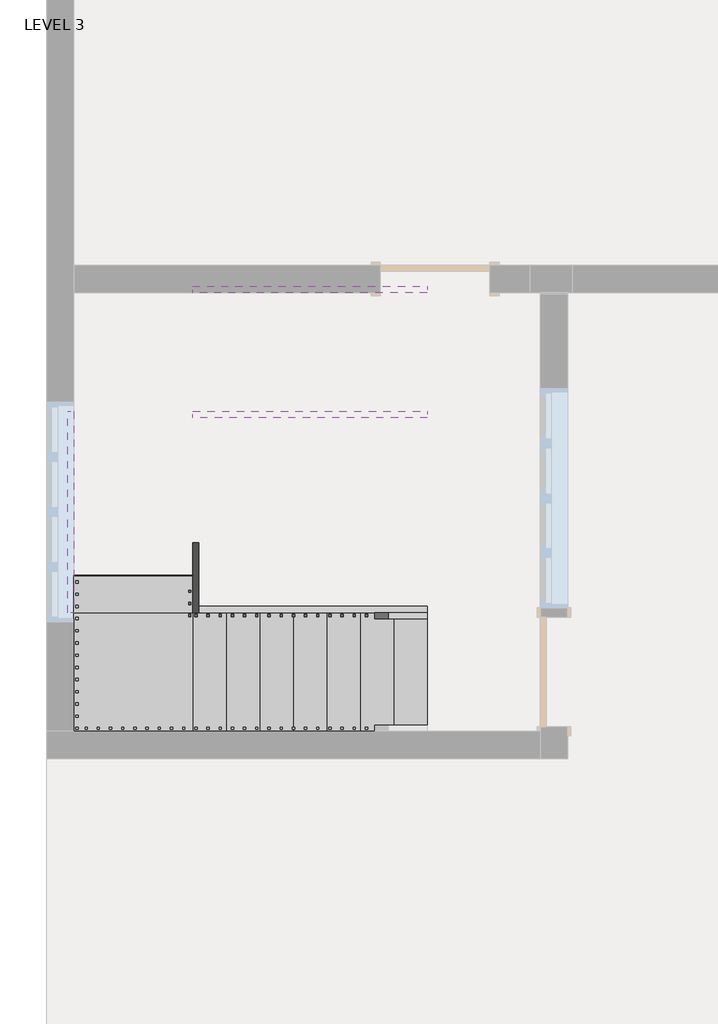
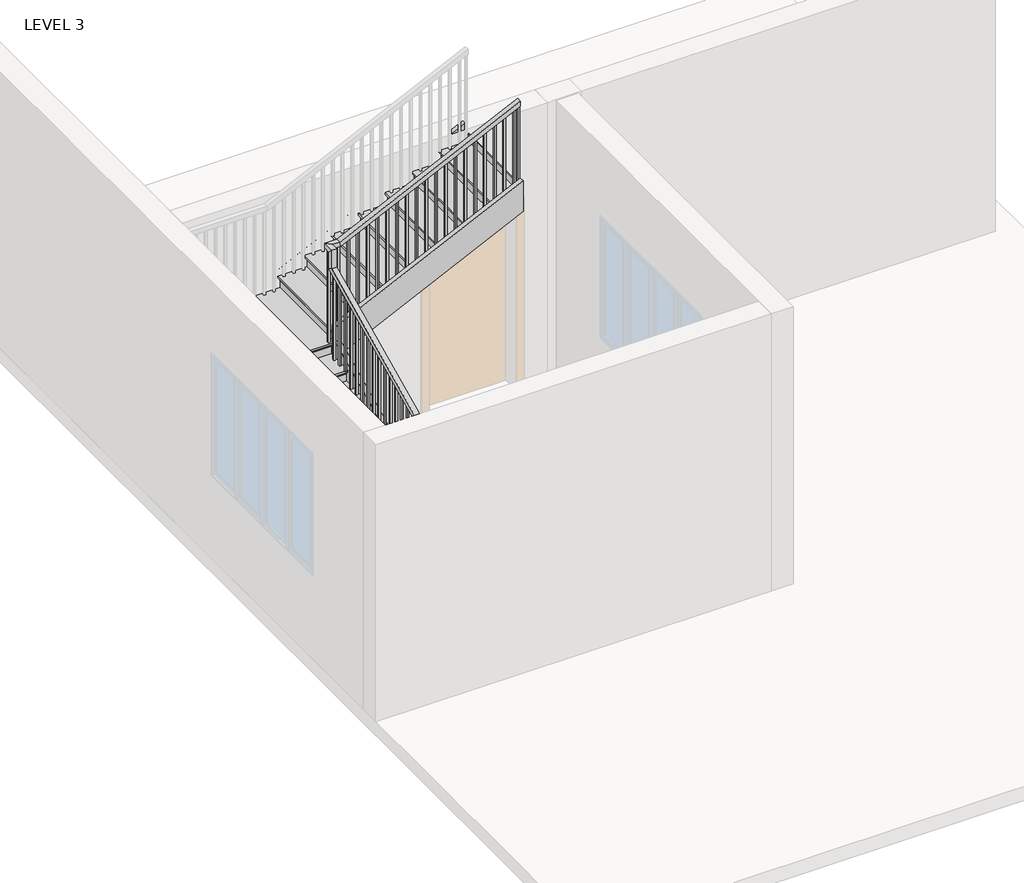
# One storey, part 3 of 3: 6 members, 1 railing, 1 stair flight.
"""IFC4 building model written with IfcOpenShell, lengths in millimetres."""

from ifc_helpers import new_model, si_unit, frame, origin, place, context, project, spatial, polyline, outline, extrude, faceted_brep, transform, mapped, element, save
from components import stair_flight_8adf14a6

model = new_model("IFC4")

# Units and contexts
model_context = context("Model", 3, world=origin())
ifc_project = project(units=[si_unit("LENGTHUNIT", "METRE", prefix="MILLI")], contexts=[model_context])

# Site, building, storey
site = spatial("IfcSite", under=ifc_project)
building = spatial("IfcBuilding", under=site)
storey = spatial("IfcBuildingStorey", under=building, Name="LEVEL 3", Elevation=6248.4)

# Members
placement = place(None, origin())
element("IfcMember", 1, ObjectType="Stringer - 2\" Width", at=placement, inside=storey, context=model_context, shape_type="SweptSolid", body=[
    extrude(outline(polyline([(6248.4, -19769.8789184), (6449.6074226, -19769.8789184), (7039.9315333, -21014.4789184), (7039.9315333, -21725.7197387), (6248.4, -20056.9074227), (6248.4, -19769.8789184)])), frame((0.0, -1169.2399287, 0.0), z_axis=(0.0, 1.0, 0.0), x_axis=(0.0, 0.0, 1.0)), (0.0, 0.0, 1.0), 50.8),
])
element("IfcMember", 2, ObjectType="Stringer - 2\" Width", at=placement, inside=storey, context=model_context, shape_type="SweptSolid", body=[
    extrude(outline(polyline([(-127.880749, 7509.7619743), (837.3600713, 7967.5837072), (1548.6008915, 7967.5837072), (583.3600713, 7509.7619743), (-127.880749, 7509.7619743)])), frame((-22767.0789184, 0.0, 0.0), z_axis=(1.0, 0.0, 0.0), x_axis=(0.0, 1.0, 0.0)), (0.0, 0.0, 1.0), 50.8),
])
element("IfcMember", 3, ObjectType="Stringer - 2\" Width", at=placement, inside=storey, context=model_context, shape_type="SweptSolid", body=[
    extrude(outline(polyline([(8437.4141482, -21014.4789184), (9027.7382589, -19769.8789184), (9365.0856835, -19769.8789184), (8437.4141482, -21725.7197387), (8437.4141482, -21014.4789184)])), frame((0.0, 2539.1600713, 0.0), z_axis=(0.0, 1.0, 0.0), x_axis=(0.0, 0.0, 1.0)), (0.0, 0.0, 1.0), 50.8),
])
element("IfcMember", 4, ObjectType="Stringer - 2\" Width", at=placement, inside=storey, context=model_context, shape_type="SweptSolid", body=[
    extrude(outline(polyline([(6248.4, -19769.8789184), (6449.6074226, -19769.8789184), (7353.1647349, -21674.8789184), (7015.8173103, -21674.8789184), (6248.4, -20056.9074227), (6248.4, -19769.8789184)])), frame((0.0, -127.8399287, 0.0), z_axis=(0.0, 1.0, 0.0), x_axis=(0.0, 0.0, 1.0)), (0.0, 0.0, 1.0), 50.8),
])
element("IfcMember", 5, ObjectType="Stringer - 2\" Width", at=placement, inside=storey, context=model_context, shape_type="SweptSolid", body=[
    extrude(outline(polyline([(-127.8399287, 7172.433911), (-127.8399287, 7509.7813357), (1497.7600713, 8280.8169088), (1497.7600713, 7943.4694842), (-127.8399287, 7172.433911)])), frame((-21725.6789184, 0.0, 0.0), z_axis=(1.0, 0.0, 0.0), x_axis=(0.0, 1.0, 0.0)), (0.0, 0.0, 1.0), 50.8),
])
element("IfcMember", 6, ObjectType="Stringer - 2\" Width", at=placement, inside=storey, context=model_context, shape_type="SweptSolid", body=[
    extrude(outline(polyline([(8437.4335096, -21725.6789184), (8100.086085, -21725.6789184), (9027.7382589, -19769.8789184), (9365.0856835, -19769.8789184), (8437.4335096, -21725.6789184)])), frame((0.0, 1497.7600713, 0.0), z_axis=(0.0, 1.0, 0.0), x_axis=(0.0, 0.0, 1.0)), (0.0, 0.0, 1.0), 50.8),
])

# Railing
element("IfcRailing", 7, ObjectType="Handrail - Rectangular", at=placement, inside=storey, context=model_context, shape_type="SolidModel", body=[
    faceted_brep([(-19769.8789184, -178.6399287, 7295.3217391), (-19769.8789184, -178.6399287, 7239.0971684), (-19769.8789184, -127.8399287, 7239.0971684), (-19769.8789184, -127.8399287, 7295.3217391), (-21649.4789184, -178.6399287, 8186.8316206), (-21700.2789184, -178.6399287, 8154.7019114), (-21700.2789184, -127.8399287, 8154.7019114), (-21649.4789184, -127.8399287, 8186.8316206), (-21776.4789184, -40.2031254, 8340.8379447), (-21776.4789184, -51.6399287, 8391.6379447), (-21776.4789184, 1472.3600713, 9114.4837945), (-21776.4789184, 1523.1600713, 9082.3540854), (-21725.6789184, -40.2031254, 8340.8379447), (-21725.6789184, 1523.1600713, 9082.3540854), (-21725.6789184, -51.6399287, 8391.6379447), (-21725.6789184, 1472.3600713, 9114.4837945), (-19769.8789184, 1599.3600713, 10210.8), (-19769.8789184, 1548.5600713, 10210.8), (-19769.8789184, 1548.5600713, 10154.5754292), (-19769.8789184, 1599.3600713, 10154.5754292), (-21638.0421151, 1599.3600713, 9268.4901186), (-21649.4789184, 1599.3600713, 9319.2901186), (-21638.0421151, 1548.5600713, 9268.4901186), (-21649.4789184, 1548.5600713, 9319.2901186), (-21649.4789184, -178.6399287, 8391.6379447), (-21700.2789184, -178.6399287, 8340.8379447), (-21700.2789184, -127.8399287, 8340.8379447), (-21649.4789184, -127.8399287, 8391.6379447), (-21776.4789184, -178.6399287, 8391.6379447), (-21776.4789184, -178.6399287, 8340.8379447), (-21725.6789184, -127.8399287, 8340.8379447), (-21725.6789184, -127.8399287, 8391.6379447), (-21776.4789184, 1472.3600713, 9319.2901186), (-21776.4789184, 1523.1600713, 9268.4901186), (-21725.6789184, 1523.1600713, 9268.4901186), (-21725.6789184, 1472.3600713, 9319.2901186), (-21776.4789184, 1599.3600713, 9319.2901186), (-21776.4789184, 1599.3600713, 9268.4901186), (-21725.6789184, 1548.5600713, 9268.4901186), (-21725.6789184, 1548.5600713, 9319.2901186)], [[[0, 1, 2, 3]], [[1, 0, 4, 5]], [[2, 1, 5, 6]], [[3, 2, 6, 7]], [[0, 3, 7, 4]], [[8, 9, 10, 11]], [[12, 8, 11, 13]], [[14, 12, 13, 15]], [[9, 14, 15, 10]], [[16, 17, 18, 19]], [[20, 21, 16, 19]], [[22, 20, 19, 18]], [[23, 22, 18, 17]], [[21, 23, 17, 16]], [[5, 4, 24, 25]], [[6, 5, 25, 26]], [[7, 6, 26, 27]], [[4, 7, 27, 24]], [[25, 24, 28, 29]], [[26, 25, 29, 30]], [[27, 26, 30, 31]], [[24, 27, 31, 28]], [[29, 28, 9, 8]], [[30, 29, 8, 12]], [[31, 30, 12, 14]], [[28, 31, 14, 9]], [[11, 10, 32, 33]], [[13, 11, 33, 34]], [[15, 13, 34, 35]], [[10, 15, 35, 32]], [[33, 32, 36, 37]], [[34, 33, 37, 38]], [[35, 34, 38, 39]], [[32, 35, 39, 36]], [[37, 36, 21, 20]], [[38, 37, 20, 22]], [[39, 38, 22, 23]], [[36, 39, 23, 21]]]),
    extrude(outline(polyline([(10134.9983541, -19811.1539184), (10125.962781, -19830.2039184), (9163.8782609, -19830.2039184), (9163.8782609, -19811.1539184), (10134.9983541, -19811.1539184)])), frame((0.0, 1564.4350713, 0.0), z_axis=(0.0, 1.0, 0.0), x_axis=(0.0, 0.0, 1.0)), (0.0, 0.0, 1.0), 19.05),
    extrude(outline(polyline([(10086.8086308, -19912.7539184), (10077.7730577, -19931.8039184), (9163.8782609, -19931.8039184), (9163.8782609, -19912.7539184), (10086.8086308, -19912.7539184)])), frame((0.0, 1564.4350713, 0.0), z_axis=(0.0, 1.0, 0.0), x_axis=(0.0, 0.0, 1.0)), (0.0, 0.0, 1.0), 19.05),
    extrude(outline(polyline([(10038.6189075, -20014.3539184), (10029.5833344, -20033.4039184), (9163.8782609, -20033.4039184), (9163.8782609, -20014.3539184), (10038.6189075, -20014.3539184)])), frame((0.0, 1564.4350713, 0.0), z_axis=(0.0, 1.0, 0.0), x_axis=(0.0, 0.0, 1.0)), (0.0, 0.0, 1.0), 19.05),
    extrude(outline(polyline([(9990.4291842, -20115.9539184), (9981.393611, -20135.0039184), (9031.3565217, -20135.0039184), (9031.3565217, -20115.9539184), (9990.4291842, -20115.9539184)])), frame((0.0, 1564.4350713, 0.0), z_axis=(0.0, 1.0, 0.0), x_axis=(0.0, 0.0, 1.0)), (0.0, 0.0, 1.0), 19.05),
    extrude(outline(polyline([(9942.2394608, -20217.5539184), (9933.2038877, -20236.6039184), (9031.3565217, -20236.6039184), (9031.3565217, -20217.5539184), (9942.2394608, -20217.5539184)])), frame((0.0, 1564.4350713, 0.0), z_axis=(0.0, 1.0, 0.0), x_axis=(0.0, 0.0, 1.0)), (0.0, 0.0, 1.0), 19.05),
    extrude(outline(polyline([(9894.0497375, -20319.1539184), (9885.0141644, -20338.2039184), (9031.3565217, -20338.2039184), (9031.3565217, -20319.1539184), (9894.0497375, -20319.1539184)])), frame((0.0, 1564.4350713, 0.0), z_axis=(0.0, 1.0, 0.0), x_axis=(0.0, 0.0, 1.0)), (0.0, 0.0, 1.0), 19.05),
    extrude(outline(polyline([(9845.8600142, -20420.7539184), (9836.8244411, -20439.8039184), (8898.8347826, -20439.8039184), (8898.8347826, -20420.7539184), (9845.8600142, -20420.7539184)])), frame((0.0, 1564.4350713, 0.0), z_axis=(0.0, 1.0, 0.0), x_axis=(0.0, 0.0, 1.0)), (0.0, 0.0, 1.0), 19.05),
    extrude(outline(polyline([(9797.6702909, -20522.3539184), (9788.6347178, -20541.4039184), (8898.8347826, -20541.4039184), (8898.8347826, -20522.3539184), (9797.6702909, -20522.3539184)])), frame((0.0, 1564.4350713, 0.0), z_axis=(0.0, 1.0, 0.0), x_axis=(0.0, 0.0, 1.0)), (0.0, 0.0, 1.0), 19.05),
    extrude(outline(polyline([(9749.4805676, -20623.9539184), (9740.4449944, -20643.0039184), (8766.3130435, -20643.0039184), (8766.3130435, -20623.9539184), (9749.4805676, -20623.9539184)])), frame((0.0, 1564.4350713, 0.0), z_axis=(0.0, 1.0, 0.0), x_axis=(0.0, 0.0, 1.0)), (0.0, 0.0, 1.0), 19.05),
    extrude(outline(polyline([(9701.2908442, -20725.5539184), (9692.2552711, -20744.6039184), (8766.3130435, -20744.6039184), (8766.3130435, -20725.5539184), (9701.2908442, -20725.5539184)])), frame((0.0, 1564.4350713, 0.0), z_axis=(0.0, 1.0, 0.0), x_axis=(0.0, 0.0, 1.0)), (0.0, 0.0, 1.0), 19.05),
    extrude(outline(polyline([(9653.1011209, -20827.1539184), (9644.0655478, -20846.2039184), (8766.3130435, -20846.2039184), (8766.3130435, -20827.1539184), (9653.1011209, -20827.1539184)])), frame((0.0, 1564.4350713, 0.0), z_axis=(0.0, 1.0, 0.0), x_axis=(0.0, 0.0, 1.0)), (0.0, 0.0, 1.0), 19.05),
    extrude(outline(polyline([(9604.9113976, -20928.7539184), (9595.8758245, -20947.8039184), (8633.7913043, -20947.8039184), (8633.7913043, -20928.7539184), (9604.9113976, -20928.7539184)])), frame((0.0, 1564.4350713, 0.0), z_axis=(0.0, 1.0, 0.0), x_axis=(0.0, 0.0, 1.0)), (0.0, 0.0, 1.0), 19.05),
    extrude(outline(polyline([(9556.7216743, -21030.3539184), (9547.6861012, -21049.4039184), (8633.7913043, -21049.4039184), (8633.7913043, -21030.3539184), (9556.7216743, -21030.3539184)])), frame((0.0, 1564.4350713, 0.0), z_axis=(0.0, 1.0, 0.0), x_axis=(0.0, 0.0, 1.0)), (0.0, 0.0, 1.0), 19.05),
    extrude(outline(polyline([(9508.531951, -21131.9539184), (9499.4963778, -21151.0039184), (8633.7913043, -21151.0039184), (8633.7913043, -21131.9539184), (9508.531951, -21131.9539184)])), frame((0.0, 1564.4350713, 0.0), z_axis=(0.0, 1.0, 0.0), x_axis=(0.0, 0.0, 1.0)), (0.0, 0.0, 1.0), 19.05),
    extrude(outline(polyline([(9460.3422276, -21233.5539184), (9451.3066545, -21252.6039184), (8501.2695652, -21252.6039184), (8501.2695652, -21233.5539184), (9460.3422276, -21233.5539184)])), frame((0.0, 1564.4350713, 0.0), z_axis=(0.0, 1.0, 0.0), x_axis=(0.0, 0.0, 1.0)), (0.0, 0.0, 1.0), 19.05),
    extrude(outline(polyline([(9412.1525043, -21335.1539184), (9403.1169312, -21354.2039184), (8501.2695652, -21354.2039184), (8501.2695652, -21335.1539184), (9412.1525043, -21335.1539184)])), frame((0.0, 1564.4350713, 0.0), z_axis=(0.0, 1.0, 0.0), x_axis=(0.0, 0.0, 1.0)), (0.0, 0.0, 1.0), 19.05),
    extrude(outline(polyline([(9363.962781, -21436.7539184), (9354.9272079, -21455.8039184), (8501.2695652, -21455.8039184), (8501.2695652, -21436.7539184), (9363.962781, -21436.7539184)])), frame((0.0, 1564.4350713, 0.0), z_axis=(0.0, 1.0, 0.0), x_axis=(0.0, 0.0, 1.0)), (0.0, 0.0, 1.0), 19.05),
    extrude(outline(polyline([(9315.7730577, -21538.3539184), (9306.7374846, -21557.4039184), (8368.7478261, -21557.4039184), (8368.7478261, -21538.3539184), (9315.7730577, -21538.3539184)])), frame((0.0, 1564.4350713, 0.0), z_axis=(0.0, 1.0, 0.0), x_axis=(0.0, 0.0, 1.0)), (0.0, 0.0, 1.0), 19.05),
    extrude(outline(polyline([(9267.5833344, -21639.9539184), (9258.5477612, -21659.0039184), (8368.7478261, -21659.0039184), (8368.7478261, -21639.9539184), (9267.5833344, -21639.9539184)])), frame((0.0, 1564.4350713, 0.0), z_axis=(0.0, 1.0, 0.0), x_axis=(0.0, 0.0, 1.0)), (0.0, 0.0, 1.0), 19.05),
    extrude(outline(polyline([(1462.8350713, 9053.7414371), (1481.8850713, 9062.7770103), (1481.8850713, 8103.7043478), (1462.8350713, 8103.7043478), (1462.8350713, 9053.7414371)])), frame((-21760.6039184, 0.0, 0.0), z_axis=(1.0, 0.0, 0.0), x_axis=(0.0, 1.0, 0.0)), (0.0, 0.0, 1.0), 19.05),
    extrude(outline(polyline([(1361.2350713, 9005.5517138), (1380.2850713, 9014.5872869), (1380.2850713, 8103.7043478), (1361.2350713, 8103.7043478), (1361.2350713, 9005.5517138)])), frame((-21760.6039184, 0.0, 0.0), z_axis=(1.0, 0.0, 0.0), x_axis=(0.0, 1.0, 0.0)), (0.0, 0.0, 1.0), 19.05),
    extrude(outline(polyline([(1259.6350713, 8957.3619905), (1278.6850713, 8966.3975636), (1278.6850713, 8103.7043478), (1259.6350713, 8103.7043478), (1259.6350713, 8957.3619905)])), frame((-21760.6039184, 0.0, 0.0), z_axis=(1.0, 0.0, 0.0), x_axis=(0.0, 1.0, 0.0)), (0.0, 0.0, 1.0), 19.05),
    extrude(outline(polyline([(1158.0350713, 8909.1722672), (1177.0850713, 8918.2078403), (1177.0850713, 7971.1826087), (1158.0350713, 7971.1826087), (1158.0350713, 8909.1722672)])), frame((-21760.6039184, 0.0, 0.0), z_axis=(1.0, 0.0, 0.0), x_axis=(0.0, 1.0, 0.0)), (0.0, 0.0, 1.0), 19.05),
    extrude(outline(polyline([(1056.4350713, 8860.9825439), (1075.4850713, 8870.018117), (1075.4850713, 7971.1826087), (1056.4350713, 7971.1826087), (1056.4350713, 8860.9825439)])), frame((-21760.6039184, 0.0, 0.0), z_axis=(1.0, 0.0, 0.0), x_axis=(0.0, 1.0, 0.0)), (0.0, 0.0, 1.0), 19.05),
    extrude(outline(polyline([(954.8350713, 8812.7928205), (973.8850713, 8821.8283937), (973.8850713, 7838.6608696), (954.8350713, 7838.6608696), (954.8350713, 8812.7928205)])), frame((-21760.6039184, 0.0, 0.0), z_axis=(1.0, 0.0, 0.0), x_axis=(0.0, 1.0, 0.0)), (0.0, 0.0, 1.0), 19.05),
    extrude(outline(polyline([(853.2350713, 8764.6030972), (872.2850713, 8773.6386703), (872.2850713, 7838.6608696), (853.2350713, 7838.6608696), (853.2350713, 8764.6030972)])), frame((-21760.6039184, 0.0, 0.0), z_axis=(1.0, 0.0, 0.0), x_axis=(0.0, 1.0, 0.0)), (0.0, 0.0, 1.0), 19.05),
    extrude(outline(polyline([(751.6350713, 8716.4133739), (770.6850713, 8725.448947), (770.6850713, 7838.6608696), (751.6350713, 7838.6608696), (751.6350713, 8716.4133739)])), frame((-21760.6039184, 0.0, 0.0), z_axis=(1.0, 0.0, 0.0), x_axis=(0.0, 1.0, 0.0)), (0.0, 0.0, 1.0), 19.05),
    extrude(outline(polyline([(650.0350713, 8668.2236506), (669.0850713, 8677.2592237), (669.0850713, 7706.1391304), (650.0350713, 7706.1391304), (650.0350713, 8668.2236506)])), frame((-21760.6039184, 0.0, 0.0), z_axis=(1.0, 0.0, 0.0), x_axis=(0.0, 1.0, 0.0)), (0.0, 0.0, 1.0), 19.05),
    extrude(outline(polyline([(548.4350713, 8620.0339273), (567.4850713, 8629.0695004), (567.4850713, 7706.1391304), (548.4350713, 7706.1391304), (548.4350713, 8620.0339273)])), frame((-21760.6039184, 0.0, 0.0), z_axis=(1.0, 0.0, 0.0), x_axis=(0.0, 1.0, 0.0)), (0.0, 0.0, 1.0), 19.05),
    extrude(outline(polyline([(446.8350713, 8571.8442039), (465.8850713, 8580.8797771), (465.8850713, 7706.1391304), (446.8350713, 7706.1391304), (446.8350713, 8571.8442039)])), frame((-21760.6039184, 0.0, 0.0), z_axis=(1.0, 0.0, 0.0), x_axis=(0.0, 1.0, 0.0)), (0.0, 0.0, 1.0), 19.05),
    extrude(outline(polyline([(345.2350713, 8523.6544806), (364.2850713, 8532.6900537), (364.2850713, 7573.6173913), (345.2350713, 7573.6173913), (345.2350713, 8523.6544806)])), frame((-21760.6039184, 0.0, 0.0), z_axis=(1.0, 0.0, 0.0), x_axis=(0.0, 1.0, 0.0)), (0.0, 0.0, 1.0), 19.05),
    extrude(outline(polyline([(243.6350713, 8475.4647573), (262.6850713, 8484.5003304), (262.6850713, 7573.6173913), (243.6350713, 7573.6173913), (243.6350713, 8475.4647573)])), frame((-21760.6039184, 0.0, 0.0), z_axis=(1.0, 0.0, 0.0), x_axis=(0.0, 1.0, 0.0)), (0.0, 0.0, 1.0), 19.05),
    extrude(outline(polyline([(142.0350713, 8427.275034), (161.0850713, 8436.3106071), (161.0850713, 7573.6173913), (142.0350713, 7573.6173913), (142.0350713, 8427.275034)])), frame((-21760.6039184, 0.0, 0.0), z_axis=(1.0, 0.0, 0.0), x_axis=(0.0, 1.0, 0.0)), (0.0, 0.0, 1.0), 19.05),
    extrude(outline(polyline([(40.4350713, 8379.0853107), (59.4850713, 8388.1208838), (59.4850713, 7441.0956522), (40.4350713, 7441.0956522), (40.4350713, 8379.0853107)])), frame((-21760.6039184, 0.0, 0.0), z_axis=(1.0, 0.0, 0.0), x_axis=(0.0, 1.0, 0.0)), (0.0, 0.0, 1.0), 19.05),
    extrude(outline(polyline([(-61.1649287, 8330.8955873), (-42.1149287, 8339.9311605), (-42.1149287, 7441.0956522), (-61.1649287, 7441.0956522), (-61.1649287, 8330.8955873)])), frame((-21760.6039184, 0.0, 0.0), z_axis=(1.0, 0.0, 0.0), x_axis=(0.0, 1.0, 0.0)), (0.0, 0.0, 1.0), 19.05),
    extrude(outline(polyline([(-21690.7539184, -143.7149287), (-21690.7539184, -162.7649287), (-21709.8039184, -162.7649287), (-21709.8039184, -143.7149287), (-21690.7539184, -143.7149287)])), frame((0.0, 0.0, 7176.0521739), z_axis=(0.0, 0.0, 1.0), x_axis=(1.0, 0.0, 0.0)), (0.0, 0.0, 1.0), 1164.7857708),
    extrude(outline(polyline([(8101.9944016, -21589.1539184), (8111.0299747, -21608.2039184), (7176.0521739, -21608.2039184), (7176.0521739, -21589.1539184), (8101.9944016, -21589.1539184)])), frame((0.0, -162.7649287, 0.0), z_axis=(0.0, 1.0, 0.0), x_axis=(0.0, 0.0, 1.0)), (0.0, 0.0, 1.0), 19.05),
    extrude(outline(polyline([(8053.8046782, -21487.5539184), (8062.8402514, -21506.6039184), (7176.0521739, -21506.6039184), (7176.0521739, -21487.5539184), (8053.8046782, -21487.5539184)])), frame((0.0, -162.7649287, 0.0), z_axis=(0.0, 1.0, 0.0), x_axis=(0.0, 0.0, 1.0)), (0.0, 0.0, 1.0), 19.05),
    extrude(outline(polyline([(8005.6149549, -21385.9539184), (8014.650528, -21405.0039184), (7043.5304348, -21405.0039184), (7043.5304348, -21385.9539184), (8005.6149549, -21385.9539184)])), frame((0.0, -162.7649287, 0.0), z_axis=(0.0, 1.0, 0.0), x_axis=(0.0, 0.0, 1.0)), (0.0, 0.0, 1.0), 19.05),
    extrude(outline(polyline([(7957.4252316, -21284.3539184), (7966.4608047, -21303.4039184), (7043.5304348, -21303.4039184), (7043.5304348, -21284.3539184), (7957.4252316, -21284.3539184)])), frame((0.0, -162.7649287, 0.0), z_axis=(0.0, 1.0, 0.0), x_axis=(0.0, 0.0, 1.0)), (0.0, 0.0, 1.0), 19.05),
    extrude(outline(polyline([(7909.2355083, -21182.7539184), (7918.2710814, -21201.8039184), (7043.5304348, -21201.8039184), (7043.5304348, -21182.7539184), (7909.2355083, -21182.7539184)])), frame((0.0, -162.7649287, 0.0), z_axis=(0.0, 1.0, 0.0), x_axis=(0.0, 0.0, 1.0)), (0.0, 0.0, 1.0), 19.05),
    extrude(outline(polyline([(7861.045785, -21081.1539184), (7870.0813581, -21100.2039184), (6911.0086957, -21100.2039184), (6911.0086957, -21081.1539184), (7861.045785, -21081.1539184)])), frame((0.0, -162.7649287, 0.0), z_axis=(0.0, 1.0, 0.0), x_axis=(0.0, 0.0, 1.0)), (0.0, 0.0, 1.0), 19.05),
    extrude(outline(polyline([(7812.8560616, -20979.5539184), (7821.8916348, -20998.6039184), (6911.0086957, -20998.6039184), (6911.0086957, -20979.5539184), (7812.8560616, -20979.5539184)])), frame((0.0, -162.7649287, 0.0), z_axis=(0.0, 1.0, 0.0), x_axis=(0.0, 0.0, 1.0)), (0.0, 0.0, 1.0), 19.05),
    extrude(outline(polyline([(7764.6663383, -20877.9539184), (7773.7019114, -20897.0039184), (6911.0086957, -20897.0039184), (6911.0086957, -20877.9539184), (7764.6663383, -20877.9539184)])), frame((0.0, -162.7649287, 0.0), z_axis=(0.0, 1.0, 0.0), x_axis=(0.0, 0.0, 1.0)), (0.0, 0.0, 1.0), 19.05),
    extrude(outline(polyline([(7716.476615, -20776.3539184), (7725.5121881, -20795.4039184), (6778.4869565, -20795.4039184), (6778.4869565, -20776.3539184), (7716.476615, -20776.3539184)])), frame((0.0, -162.7649287, 0.0), z_axis=(0.0, 1.0, 0.0), x_axis=(0.0, 0.0, 1.0)), (0.0, 0.0, 1.0), 19.05),
    extrude(outline(polyline([(7668.2868917, -20674.7539184), (7677.3224648, -20693.8039184), (6778.4869565, -20693.8039184), (6778.4869565, -20674.7539184), (7668.2868917, -20674.7539184)])), frame((0.0, -162.7649287, 0.0), z_axis=(0.0, 1.0, 0.0), x_axis=(0.0, 0.0, 1.0)), (0.0, 0.0, 1.0), 19.05),
    extrude(outline(polyline([(7620.0971684, -20573.1539184), (7629.1327415, -20592.2039184), (6645.9652174, -20592.2039184), (6645.9652174, -20573.1539184), (7620.0971684, -20573.1539184)])), frame((0.0, -162.7649287, 0.0), z_axis=(0.0, 1.0, 0.0), x_axis=(0.0, 0.0, 1.0)), (0.0, 0.0, 1.0), 19.05),
    extrude(outline(polyline([(7571.907445, -20471.5539184), (7580.9430182, -20490.6039184), (6645.9652174, -20490.6039184), (6645.9652174, -20471.5539184), (7571.907445, -20471.5539184)])), frame((0.0, -162.7649287, 0.0), z_axis=(0.0, 1.0, 0.0), x_axis=(0.0, 0.0, 1.0)), (0.0, 0.0, 1.0), 19.05),
    extrude(outline(polyline([(7523.7177217, -20369.9539184), (7532.7532948, -20389.0039184), (6645.9652174, -20389.0039184), (6645.9652174, -20369.9539184), (7523.7177217, -20369.9539184)])), frame((0.0, -162.7649287, 0.0), z_axis=(0.0, 1.0, 0.0), x_axis=(0.0, 0.0, 1.0)), (0.0, 0.0, 1.0), 19.05),
    extrude(outline(polyline([(7475.5279984, -20268.3539184), (7484.5635715, -20287.4039184), (6513.4434783, -20287.4039184), (6513.4434783, -20268.3539184), (7475.5279984, -20268.3539184)])), frame((0.0, -162.7649287, 0.0), z_axis=(0.0, 1.0, 0.0), x_axis=(0.0, 0.0, 1.0)), (0.0, 0.0, 1.0), 19.05),
    extrude(outline(polyline([(7427.3382751, -20166.7539184), (7436.3738482, -20185.8039184), (6513.4434783, -20185.8039184), (6513.4434783, -20166.7539184), (7427.3382751, -20166.7539184)])), frame((0.0, -162.7649287, 0.0), z_axis=(0.0, 1.0, 0.0), x_axis=(0.0, 0.0, 1.0)), (0.0, 0.0, 1.0), 19.05),
    extrude(outline(polyline([(7379.1485518, -20065.1539184), (7388.1841249, -20084.2039184), (6513.4434783, -20084.2039184), (6513.4434783, -20065.1539184), (7379.1485518, -20065.1539184)])), frame((0.0, -162.7649287, 0.0), z_axis=(0.0, 1.0, 0.0), x_axis=(0.0, 0.0, 1.0)), (0.0, 0.0, 1.0), 19.05),
    extrude(outline(polyline([(7330.9588284, -19963.5539184), (7339.9944016, -19982.6039184), (6380.9217391, -19982.6039184), (6380.9217391, -19963.5539184), (7330.9588284, -19963.5539184)])), frame((0.0, -162.7649287, 0.0), z_axis=(0.0, 1.0, 0.0), x_axis=(0.0, 0.0, 1.0)), (0.0, 0.0, 1.0), 19.05),
    extrude(outline(polyline([(7282.7691051, -19861.9539184), (7291.8046782, -19881.0039184), (6380.9217391, -19881.0039184), (6380.9217391, -19861.9539184), (7282.7691051, -19861.9539184)])), frame((0.0, -162.7649287, 0.0), z_axis=(0.0, 1.0, 0.0), x_axis=(0.0, 0.0, 1.0)), (0.0, 0.0, 1.0), 19.05),
    extrude(outline(polyline([(-21741.5539184, 1564.4350713), (-21760.6039184, 1564.4350713), (-21760.6039184, 1583.4850713), (-21741.5539184, 1583.4850713), (-21741.5539184, 1564.4350713)])), frame((0.0, 0.0, 8236.226087), z_axis=(0.0, 0.0, 1.0), x_axis=(1.0, 0.0, 0.0)), (0.0, 0.0, 1.0), 1032.2640316),
    extrude(outline(polyline([(-21741.5539184, -143.7149287), (-21741.5539184, -162.7649287), (-21760.6039184, -162.7649287), (-21760.6039184, -143.7149287), (-21741.5539184, -143.7149287)])), frame((0.0, 0.0, 7308.573913), z_axis=(0.0, 0.0, 1.0), x_axis=(1.0, 0.0, 0.0)), (0.0, 0.0, 1.0), 1032.2640316),
    extrude(outline(polyline([(10154.5754292, -19769.8789184), (10145.5398561, -19788.9289184), (9163.8782609, -19788.9289184), (9163.8782609, -19769.8789184), (10154.5754292, -19769.8789184)])), frame((0.0, 1564.4350713, 0.0), z_axis=(0.0, 1.0, 0.0), x_axis=(0.0, 0.0, 1.0)), (0.0, 0.0, 1.0), 19.05),
    extrude(outline(polyline([(7239.0971684, -19769.8789184), (7248.1327415, -19788.9289184), (6380.9217391, -19788.9289184), (6380.9217391, -19769.8789184), (7239.0971684, -19769.8789184)])), frame((0.0, -162.7649287, 0.0), z_axis=(0.0, 1.0, 0.0), x_axis=(0.0, 0.0, 1.0)), (0.0, 0.0, 1.0), 19.05),
])

# Stair flight
stair_flight_shape = stair_flight_8adf14a6(model_context)
element("IfcStairFlight", 8, ObjectType="2\" Tread 1\" Nosing 1/4\" Riser", at=placement, inside=storey, context=model_context, shape_type="MappedRepresentation", body=[
    mapped(stair_flight_shape, transform((0.0, 0.0, 0.0), x_axis=(1.0, 0.0, 0.0), y_axis=(0.0, 1.0, 0.0), z_axis=(0.0, 0.0, 1.0))),
])

save(model, "model.ifc")

# Revit data of these elements
# Type "Handrail - Rectangular"
#   Assembly Code = "C2010400"
#   built-in parameter 1008612 = 0.0416667 (stored number, unit not read)
#   built-in parameter 1008611 = 0.0416667 (stored number, unit not read)
#   built-in parameter 1008609 = 0.333333 (stored number, unit not read)
#   built-in parameter 1008604 = 0.166667 (stored number, unit not read)
#   built-in parameter 1008603 = 0.166667 (stored number, unit not read)
#   Railing Height = 3' - 0"
#   built-in parameter 1008630 = 2
#   built-in parameter 1008610 = 2
#   built-in parameter 1008618 = Baluster - Square : 3/4"
# Elements 1, 2, 3, 4, 5, 6 (IfcMember, "Stringer - 2\" Width")
#   Phase Created = New Construction
# Element 7 (IfcRailing, "Handrail - Rectangular")
#   Phase Created = New Construction
# Element 8 (IfcStairFlight, "2\" Tread 1\" Nosing 1/4\" Riser")
#   Phase Created = New Construction
